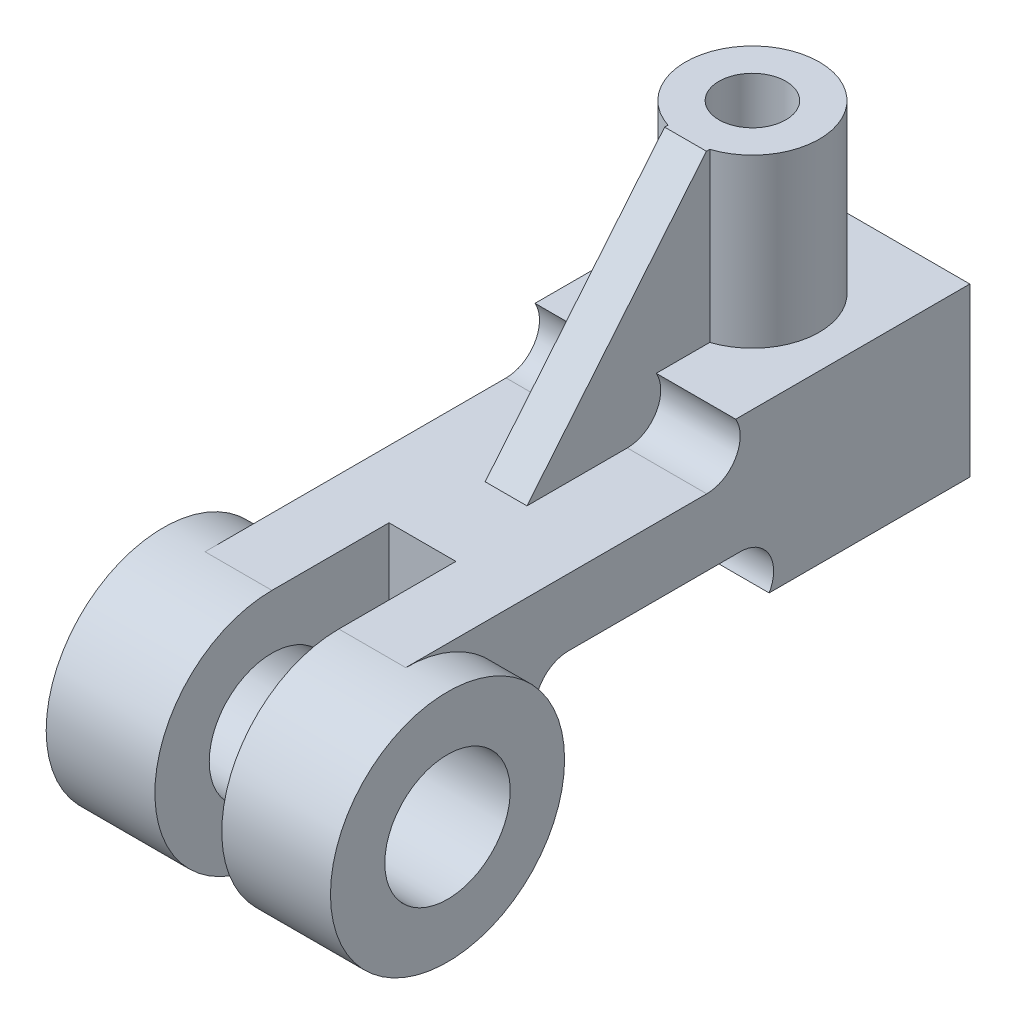
ISO-10303-21;
HEADER;
FILE_DESCRIPTION(('STEP AP214'),'2;1');
FILE_NAME('part.step','',(''),(''),'','','');
FILE_SCHEMA(('AUTOMOTIVE_DESIGN { 1 0 10303 214 1 1 1 1 }'));
ENDSEC;
DATA;
#1=APPLICATION_CONTEXT('core data for automotive mechanical design processes');
#2=APPLICATION_PROTOCOL_DEFINITION('international standard','automotive_design',2000,#1);
#3=PRODUCT_CONTEXT('',#1,'mechanical');
#4=PRODUCT('Part','Part','',(#3));
#5=PRODUCT_RELATED_PRODUCT_CATEGORY('part','',(#4));
#6=PRODUCT_DEFINITION_FORMATION('','',#4);
#7=PRODUCT_DEFINITION_CONTEXT('part definition',#1,'design');
#8=PRODUCT_DEFINITION('design','',#6,#7);
#9=PRODUCT_DEFINITION_SHAPE('','',#8);
#10=(LENGTH_UNIT() NAMED_UNIT(*) SI_UNIT(.MILLI.,.METRE.));
#11=(NAMED_UNIT(*) PLANE_ANGLE_UNIT() SI_UNIT($,.RADIAN.));
#12=(NAMED_UNIT(*) SI_UNIT($,.STERADIAN.) SOLID_ANGLE_UNIT());
#13=UNCERTAINTY_MEASURE_WITH_UNIT(LENGTH_MEASURE(1.E-05),#10,'distance_accuracy_value','');
#14=(GEOMETRIC_REPRESENTATION_CONTEXT(3) GLOBAL_UNCERTAINTY_ASSIGNED_CONTEXT((#13)) GLOBAL_UNIT_ASSIGNED_CONTEXT((#10,
#11,#12)) REPRESENTATION_CONTEXT('',''));
#15=CARTESIAN_POINT('',(0.,0.,0.));
#16=DIRECTION('',(0.,0.,1.));
#17=DIRECTION('',(1.,0.,0.));
#18=AXIS2_PLACEMENT_3D('',#15,#16,#17);
#19=CARTESIAN_POINT('',(-16.,28.,0.));
#20=DIRECTION('',(0.,-1.,0.));
#21=DIRECTION('',(0.,0.,-1.));
#22=AXIS2_PLACEMENT_3D('',#19,#20,#21);
#23=PLANE('',#22);
#24=DIRECTION('',(0.,0.,-1.));
#25=VECTOR('',#24,1.);
#26=CARTESIAN_POINT('',(-3.,28.,-72.0000000000001));
#27=LINE('',#26,#25);
#28=CARTESIAN_POINT('',(-3.,28.,-48.));
#29=VERTEX_POINT('',#28);
#30=CARTESIAN_POINT('',(-3.,28.,-72.0000000000001));
#31=VERTEX_POINT('',#30);
#32=EDGE_CURVE('E205',#29,#31,#27,.T.);
#33=ORIENTED_EDGE('',*,*,#32,.F.);
#34=DIRECTION('',(-1.,0.,0.));
#35=VECTOR('',#34,1.);
#36=CARTESIAN_POINT('',(-3.,28.,-48.));
#37=LINE('',#36,#35);
#38=CARTESIAN_POINT('',(-13.,28.,-48.));
#39=VERTEX_POINT('',#38);
#40=EDGE_CURVE('E199',#29,#39,#37,.T.);
#41=ORIENTED_EDGE('',*,*,#40,.T.);
#42=DIRECTION('',(0.,0.,-1.));
#43=VECTOR('',#42,1.);
#44=CARTESIAN_POINT('',(-13.,28.,-72.0000000000001));
#45=LINE('',#44,#43);
#46=CARTESIAN_POINT('',(-13.,28.,-72.0000000000001));
#47=VERTEX_POINT('',#46);
#48=EDGE_CURVE('E365',#39,#47,#45,.T.);
#49=ORIENTED_EDGE('',*,*,#48,.T.);
#50=DIRECTION('',(1.,0.,0.));
#51=VECTOR('',#50,1.);
#52=CARTESIAN_POINT('',(-16.,28.,-71.9999999999999));
#53=LINE('',#52,#51);
#54=CARTESIAN_POINT('',(-32.,28.,-72.));
#55=VERTEX_POINT('',#54);
#56=EDGE_CURVE('E332',#55,#47,#53,.T.);
#57=ORIENTED_EDGE('',*,*,#56,.F.);
#58=DIRECTION('',(0.,0.,-1.));
#59=VECTOR('',#58,1.);
#60=CARTESIAN_POINT('',(-32.,28.,0.));
#61=LINE('',#60,#59);
#62=CARTESIAN_POINT('',(-32.,28.,0.));
#63=VERTEX_POINT('',#62);
#64=EDGE_CURVE('E264',#63,#55,#61,.T.);
#65=ORIENTED_EDGE('',*,*,#64,.F.);
#66=DIRECTION('',(1.,0.,0.));
#67=VECTOR('',#66,1.);
#68=CARTESIAN_POINT('',(-32.,28.,0.));
#69=LINE('',#68,#67);
#70=CARTESIAN_POINT('',(-16.,28.,0.));
#71=VERTEX_POINT('',#70);
#72=EDGE_CURVE('E272',#63,#71,#69,.T.);
#73=ORIENTED_EDGE('',*,*,#72,.T.);
#74=DIRECTION('',(0.,0.,1.));
#75=VECTOR('',#74,1.);
#76=CARTESIAN_POINT('',(-16.,28.,0.));
#77=LINE('',#76,#75);
#78=CARTESIAN_POINT('',(-16.,28.,-28.));
#79=VERTEX_POINT('',#78);
#80=EDGE_CURVE('E240',#79,#71,#77,.T.);
#81=ORIENTED_EDGE('',*,*,#80,.F.);
#82=DIRECTION('',(-1.,0.,0.));
#83=VECTOR('',#82,1.);
#84=CARTESIAN_POINT('',(-16.,28.,-28.));
#85=LINE('',#84,#83);
#86=CARTESIAN_POINT('',(0.,28.,-28.));
#87=VERTEX_POINT('',#86);
#88=EDGE_CURVE('E233',#87,#79,#85,.T.);
#89=ORIENTED_EDGE('',*,*,#88,.F.);
#90=DIRECTION('',(0.,0.,-1.));
#91=VECTOR('',#90,1.);
#92=CARTESIAN_POINT('',(0.,28.,0.));
#93=LINE('',#92,#91);
#94=CARTESIAN_POINT('',(0.,28.,0.));
#95=VERTEX_POINT('',#94);
#96=EDGE_CURVE('E227',#95,#87,#93,.T.);
#97=ORIENTED_EDGE('',*,*,#96,.F.);
#98=DIRECTION('',(1.,0.,0.));
#99=VECTOR('',#98,1.);
#100=CARTESIAN_POINT('',(-16.,28.,0.));
#101=LINE('',#100,#99);
#102=CARTESIAN_POINT('',(16.,28.,0.));
#103=VERTEX_POINT('',#102);
#104=EDGE_CURVE('E331',#95,#103,#101,.T.);
#105=ORIENTED_EDGE('',*,*,#104,.T.);
#106=DIRECTION('',(0.,0.,-1.));
#107=VECTOR('',#106,1.);
#108=CARTESIAN_POINT('',(16.,28.,0.));
#109=LINE('',#108,#107);
#110=CARTESIAN_POINT('',(16.,28.,-71.9999999999999));
#111=VERTEX_POINT('',#110);
#112=EDGE_CURVE('E288',#103,#111,#109,.T.);
#113=ORIENTED_EDGE('',*,*,#112,.T.);
#114=EDGE_CURVE('E329',#31,#111,#53,.T.);
#115=ORIENTED_EDGE('',*,*,#114,.F.);
#116=EDGE_LOOP('',(#33,#41,#49,#57,#65,#73,#81,#89,#97,#105,#113,#115));
#117=FACE_BOUND('',#116,.T.);
#118=ADVANCED_FACE('F50',(#117),#23,.F.);
#119=CARTESIAN_POINT('',(-16.,36.,-72.));
#120=DIRECTION('',(1.,0.,0.));
#121=DIRECTION('',(0.,0.,-1.));
#122=AXIS2_PLACEMENT_3D('',#119,#120,#121);
#123=CYLINDRICAL_SURFACE('',#122,7.99999999999999);
#124=CARTESIAN_POINT('',(-3.,36.,-72.));
#125=DIRECTION('',(1.,0.,0.));
#126=DIRECTION('',(0.,0.,1.));
#127=AXIS2_PLACEMENT_3D('',#124,#125,#126);
#128=CIRCLE('',#127,8.);
#129=CARTESIAN_POINT('',(-3.,40.,-78.9282032302755));
#130=VERTEX_POINT('',#129);
#131=EDGE_CURVE('E373',#31,#130,#128,.T.);
#132=ORIENTED_EDGE('',*,*,#131,.F.);
#133=ORIENTED_EDGE('',*,*,#114,.T.);
#134=CARTESIAN_POINT('',(16.,36.,-72.));
#135=DIRECTION('',(1.,0.,0.));
#136=DIRECTION('',(0.,0.,-1.));
#137=AXIS2_PLACEMENT_3D('',#134,#135,#136);
#138=CIRCLE('',#137,7.99999999999999);
#139=CARTESIAN_POINT('',(16.,40.,-78.9282032302755));
#140=VERTEX_POINT('',#139);
#141=EDGE_CURVE('E291',#111,#140,#138,.T.);
#142=ORIENTED_EDGE('',*,*,#141,.T.);
#143=DIRECTION('',(1.,0.,0.));
#144=VECTOR('',#143,1.);
#145=CARTESIAN_POINT('',(-16.,40.,-78.9282032302755));
#146=LINE('',#145,#144);
#147=EDGE_CURVE('E326',#130,#140,#146,.T.);
#148=ORIENTED_EDGE('',*,*,#147,.F.);
#149=EDGE_LOOP('',(#132,#133,#142,#148));
#150=FACE_BOUND('',#149,.T.);
#151=ADVANCED_FACE('F379',(#150),#123,.F.);
#152=CARTESIAN_POINT('',(-16.,40.,-78.9282032302755));
#153=DIRECTION('',(0.,-1.,0.));
#154=DIRECTION('',(0.,0.,-1.));
#155=AXIS2_PLACEMENT_3D('',#152,#153,#154);
#156=PLANE('',#155);
#157=DIRECTION('',(0.,0.,-1.));
#158=VECTOR('',#157,1.);
#159=CARTESIAN_POINT('',(-3.,40.,-93.4436906240122));
#160=LINE('',#159,#158);
#161=CARTESIAN_POINT('',(-3.,40.,-91.7295190767049));
#162=VERTEX_POINT('',#161);
#163=EDGE_CURVE('E211',#130,#162,#160,.T.);
#164=ORIENTED_EDGE('',*,*,#163,.F.);
#165=ORIENTED_EDGE('',*,*,#147,.T.);
#166=DIRECTION('',(0.,0.,-1.));
#167=VECTOR('',#166,1.);
#168=CARTESIAN_POINT('',(16.,40.,-78.9282032302755));
#169=LINE('',#168,#167);
#170=CARTESIAN_POINT('',(16.,40.,-134.928203230276));
#171=VERTEX_POINT('',#170);
#172=EDGE_CURVE('E298',#140,#171,#169,.T.);
#173=ORIENTED_EDGE('',*,*,#172,.T.);
#174=DIRECTION('',(1.,0.,0.));
#175=VECTOR('',#174,1.);
#176=CARTESIAN_POINT('',(-32.,40.,-134.928203230276));
#177=LINE('',#176,#175);
#178=CARTESIAN_POINT('',(-32.,40.,-134.928203230276));
#179=VERTEX_POINT('',#178);
#180=EDGE_CURVE('E224',#179,#171,#177,.T.);
#181=ORIENTED_EDGE('',*,*,#180,.F.);
#182=DIRECTION('',(0.,0.,1.));
#183=VECTOR('',#182,1.);
#184=CARTESIAN_POINT('',(-32.,40.,0.));
#185=LINE('',#184,#183);
#186=CARTESIAN_POINT('',(-32.,40.,-78.9282032302755));
#187=VERTEX_POINT('',#186);
#188=EDGE_CURVE('E257',#179,#187,#185,.T.);
#189=ORIENTED_EDGE('',*,*,#188,.T.);
#190=CARTESIAN_POINT('',(-13.,40.,-78.9282032302755));
#191=VERTEX_POINT('',#190);
#192=EDGE_CURVE('E330',#187,#191,#146,.T.);
#193=ORIENTED_EDGE('',*,*,#192,.T.);
#194=DIRECTION('',(0.,0.,-1.));
#195=VECTOR('',#194,1.);
#196=CARTESIAN_POINT('',(-13.,40.,-93.4436906240122));
#197=LINE('',#196,#195);
#198=CARTESIAN_POINT('',(-13.,40.,-91.7295190767049));
#199=VERTEX_POINT('',#198);
#200=EDGE_CURVE('E193',#191,#199,#197,.T.);
#201=ORIENTED_EDGE('',*,*,#200,.T.);
#202=CARTESIAN_POINT('',(-8.,40.,-106.928203230276));
#203=DIRECTION('',(0.,-1.,0.));
#204=DIRECTION('',(0.,0.,-1.));
#205=AXIS2_PLACEMENT_3D('',#202,#203,#204);
#206=CIRCLE('',#205,16.);
#207=EDGE_CURVE('E348',#162,#199,#206,.F.);
#208=ORIENTED_EDGE('',*,*,#207,.F.);
#209=EDGE_LOOP('',(#164,#165,#173,#181,#189,#193,#201,#208));
#210=FACE_BOUND('',#209,.T.);
#211=ADVANCED_FACE('F363',(#210),#156,.F.);
#212=CARTESIAN_POINT('',(-8.,80.,-106.928203230276));
#213=DIRECTION('',(0.,-1.,0.));
#214=DIRECTION('',(0.,0.,-1.));
#215=AXIS2_PLACEMENT_3D('',#212,#213,#214);
#216=CYLINDRICAL_SURFACE('',#215,16.);
#217=DIRECTION('',(0.,-1.,0.));
#218=VECTOR('',#217,1.);
#219=CARTESIAN_POINT('',(-3.,80.,-91.7295190767049));
#220=LINE('',#219,#218);
#221=CARTESIAN_POINT('',(-3.,80.,-91.7295190767049));
#222=VERTEX_POINT('',#221);
#223=EDGE_CURVE('E11',#162,#222,#220,.F.);
#224=ORIENTED_EDGE('',*,*,#223,.F.);
#225=ORIENTED_EDGE('',*,*,#207,.T.);
#226=DIRECTION('',(0.,-1.,0.));
#227=VECTOR('',#226,1.);
#228=CARTESIAN_POINT('',(-13.,80.,-91.7295190767049));
#229=LINE('',#228,#227);
#230=CARTESIAN_POINT('',(-13.,80.,-91.7295190767049));
#231=VERTEX_POINT('',#230);
#232=EDGE_CURVE('E54',#199,#231,#229,.F.);
#233=ORIENTED_EDGE('',*,*,#232,.T.);
#234=CARTESIAN_POINT('',(-8.,80.,-106.928203230276));
#235=DIRECTION('',(0.,1.,0.));
#236=DIRECTION('',(0.,0.,1.));
#237=AXIS2_PLACEMENT_3D('',#234,#235,#236);
#238=CIRCLE('',#237,16.);
#239=EDGE_CURVE('E220',#222,#231,#238,.T.);
#240=ORIENTED_EDGE('',*,*,#239,.F.);
#241=EDGE_LOOP('',(#224,#225,#233,#240));
#242=FACE_BOUND('',#241,.T.);
#243=ADVANCED_FACE('F352',(#242),#216,.T.);
#244=CARTESIAN_POINT('',(26.,0.,0.));
#245=DIRECTION('',(-1.,0.,0.));
#246=DIRECTION('',(0.,0.,1.));
#247=AXIS2_PLACEMENT_3D('',#244,#245,#246);
#248=CYLINDRICAL_SURFACE('',#247,15.);
#249=CARTESIAN_POINT('',(0.,0.,0.));
#250=DIRECTION('',(1.,0.,0.));
#251=DIRECTION('',(0.,0.,-1.));
#252=AXIS2_PLACEMENT_3D('',#249,#250,#251);
#253=CIRCLE('',#252,15.);
#254=CARTESIAN_POINT('',(0.,0.,15.));
#255=VERTEX_POINT('',#254);
#256=EDGE_CURVE('E339',#255,#255,#253,.T.);
#257=CARTESIAN_POINT('',(26.,0.,0.));
#258=DIRECTION('',(1.,0.,0.));
#259=DIRECTION('',(0.,0.,-1.));
#260=AXIS2_PLACEMENT_3D('',#257,#258,#259);
#261=CIRCLE('',#260,15.);
#262=CARTESIAN_POINT('',(26.,0.,15.));
#263=VERTEX_POINT('',#262);
#264=EDGE_CURVE('E341',#263,#263,#261,.T.);
#265=CARTESIAN_POINT('',(0.,0.,15.));
#266=CARTESIAN_POINT('',(0.270833333333333,0.,15.));
#267=CARTESIAN_POINT('',(0.541666666666667,0.,15.));
#268=CARTESIAN_POINT('',(1.08333333333333,0.,15.));
#269=CARTESIAN_POINT('',(1.35416666666667,0.,15.));
#270=CARTESIAN_POINT('',(1.89583333333333,0.,15.));
#271=CARTESIAN_POINT('',(2.16666666666667,0.,15.));
#272=CARTESIAN_POINT('',(2.70833333333333,0.,15.));
#273=CARTESIAN_POINT('',(2.97916666666667,0.,15.));
#274=CARTESIAN_POINT('',(3.52083333333333,0.,15.));
#275=CARTESIAN_POINT('',(3.79166666666667,0.,15.));
#276=CARTESIAN_POINT('',(4.33333333333333,0.,15.));
#277=CARTESIAN_POINT('',(4.60416666666667,0.,15.));
#278=CARTESIAN_POINT('',(5.14583333333333,0.,15.));
#279=CARTESIAN_POINT('',(5.41666666666667,0.,15.));
#280=CARTESIAN_POINT('',(5.95833333333333,0.,15.));
#281=CARTESIAN_POINT('',(6.22916666666667,0.,15.));
#282=CARTESIAN_POINT('',(6.77083333333333,0.,15.));
#283=CARTESIAN_POINT('',(7.04166666666667,0.,15.));
#284=CARTESIAN_POINT('',(7.58333333333333,0.,15.));
#285=CARTESIAN_POINT('',(7.85416666666667,0.,15.));
#286=CARTESIAN_POINT('',(8.39583333333333,0.,15.));
#287=CARTESIAN_POINT('',(8.66666666666667,0.,15.));
#288=CARTESIAN_POINT('',(9.20833333333333,0.,15.));
#289=CARTESIAN_POINT('',(9.47916666666667,0.,15.));
#290=CARTESIAN_POINT('',(10.0208333333333,0.,15.));
#291=CARTESIAN_POINT('',(10.2916666666667,0.,15.));
#292=CARTESIAN_POINT('',(10.8333333333333,0.,15.));
#293=CARTESIAN_POINT('',(11.1041666666667,0.,15.));
#294=CARTESIAN_POINT('',(11.6458333333333,0.,15.));
#295=CARTESIAN_POINT('',(11.9166666666667,0.,15.));
#296=CARTESIAN_POINT('',(12.4583333333333,0.,15.));
#297=CARTESIAN_POINT('',(12.7291666666667,0.,15.));
#298=CARTESIAN_POINT('',(13.2708333333333,0.,15.));
#299=CARTESIAN_POINT('',(13.5416666666667,0.,15.));
#300=CARTESIAN_POINT('',(14.0833333333333,0.,15.));
#301=CARTESIAN_POINT('',(14.3541666666667,0.,15.));
#302=CARTESIAN_POINT('',(14.8958333333333,0.,15.));
#303=CARTESIAN_POINT('',(15.1666666666667,0.,15.));
#304=CARTESIAN_POINT('',(15.7083333333333,0.,15.));
#305=CARTESIAN_POINT('',(15.9791666666667,0.,15.));
#306=CARTESIAN_POINT('',(16.5208333333333,0.,15.));
#307=CARTESIAN_POINT('',(16.7916666666667,0.,15.));
#308=CARTESIAN_POINT('',(17.3333333333333,0.,15.));
#309=CARTESIAN_POINT('',(17.6041666666667,0.,15.));
#310=CARTESIAN_POINT('',(18.1458333333333,0.,15.));
#311=CARTESIAN_POINT('',(18.4166666666667,0.,15.));
#312=CARTESIAN_POINT('',(18.9583333333333,0.,15.));
#313=CARTESIAN_POINT('',(19.2291666666667,0.,15.));
#314=CARTESIAN_POINT('',(19.7708333333333,0.,15.));
#315=CARTESIAN_POINT('',(20.0416666666667,0.,15.));
#316=CARTESIAN_POINT('',(20.5833333333333,0.,15.));
#317=CARTESIAN_POINT('',(20.8541666666667,0.,15.));
#318=CARTESIAN_POINT('',(21.3958333333333,0.,15.));
#319=CARTESIAN_POINT('',(21.6666666666667,0.,15.));
#320=CARTESIAN_POINT('',(22.2083333333333,0.,15.));
#321=CARTESIAN_POINT('',(22.4791666666667,0.,15.));
#322=CARTESIAN_POINT('',(23.0208333333333,0.,15.));
#323=CARTESIAN_POINT('',(23.2916666666667,0.,15.));
#324=CARTESIAN_POINT('',(23.8333333333333,0.,15.));
#325=CARTESIAN_POINT('',(24.1041666666667,0.,15.));
#326=CARTESIAN_POINT('',(24.6458333333333,0.,15.));
#327=CARTESIAN_POINT('',(24.9166666666667,0.,15.));
#328=CARTESIAN_POINT('',(25.4583333333333,0.,15.));
#329=CARTESIAN_POINT('',(25.7291666666667,0.,15.));
#330=CARTESIAN_POINT('',(26.,0.,15.));
#331=B_SPLINE_CURVE_WITH_KNOTS('',3,(#265,#266,#267,#268,#269,#270,#271,#272,#273,#274,#275,
#276,#277,#278,#279,#280,#281,#282,#283,#284,#285,#286,#287,#288,#289,#290,#291,#292,#293,#294,
#295,#296,#297,#298,#299,#300,#301,#302,#303,#304,#305,#306,#307,#308,#309,#310,#311,#312,#313,
#314,#315,#316,#317,#318,#319,#320,#321,#322,#323,#324,#325,#326,#327,#328,#329,#330),
.UNSPECIFIED.,.F.,.F.,(4,2,2,2,2,2,2,2,2,2,2,2,2,2,2,2,2,2,2,2,2,2,2,2,2,2,2,2,2,2,2,2,4),(0.,
0.812500000000001,1.625,2.4375,3.25,4.0625,4.875,5.6875,6.5,7.3125,8.125,8.9375,9.75,10.5625,
11.375,12.1875,13.,13.8125,14.625,15.4375,16.25,17.0625,17.875,18.6875,19.5,20.3125,21.125,
21.9375,22.75,23.5625,24.375,25.1875,26.),.UNSPECIFIED.);
#332=EDGE_CURVE('BSEAM462',#255,#263,#331,.T.);
#333=ORIENTED_EDGE('',*,*,#256,.F.);
#334=ORIENTED_EDGE('',*,*,#264,.T.);
#335=ORIENTED_EDGE('',*,*,#332,.T.);
#336=ORIENTED_EDGE('',*,*,#332,.F.);
#337=EDGE_LOOP('',(#333,#335,#334,#336));
#338=FACE_BOUND('',#337,.T.);
#339=ADVANCED_FACE('F462',(#338),#248,.F.);
#340=CARTESIAN_POINT('',(0.,0.,0.));
#341=DIRECTION('',(1.,0.,0.));
#342=DIRECTION('',(0.,0.,-1.));
#343=AXIS2_PLACEMENT_3D('',#340,#341,#342);
#344=PLANE('',#343);
#345=DIRECTION('',(0.,1.,0.));
#346=VECTOR('',#345,1.);
#347=CARTESIAN_POINT('',(0.,-4.,-28.));
#348=LINE('',#347,#346);
#349=CARTESIAN_POINT('',(0.,0.,-28.));
#350=VERTEX_POINT('',#349);
#351=EDGE_CURVE('E239',#350,#87,#348,.T.);
#352=ORIENTED_EDGE('',*,*,#351,.F.);
#353=CARTESIAN_POINT('',(0.,0.,0.));
#354=DIRECTION('',(1.,0.,0.));
#355=DIRECTION('',(0.,0.,-1.));
#356=AXIS2_PLACEMENT_3D('',#353,#354,#355);
#357=CIRCLE('',#356,28.);
#358=EDGE_CURVE('E343',#95,#350,#357,.T.);
#359=ORIENTED_EDGE('',*,*,#358,.F.);
#360=ORIENTED_EDGE('',*,*,#96,.T.);
#361=EDGE_LOOP('',(#352,#359,#360));
#362=FACE_BOUND('',#361,.T.);
#363=ORIENTED_EDGE('',*,*,#256,.T.);
#364=EDGE_LOOP('',(#363));
#365=FACE_BOUND('',#364,.T.);
#366=ADVANCED_FACE('F423',(#362,#365),#344,.F.);
#367=CARTESIAN_POINT('',(26.,0.,0.));
#368=DIRECTION('',(1.,0.,0.));
#369=DIRECTION('',(0.,0.,-1.));
#370=AXIS2_PLACEMENT_3D('',#367,#368,#369);
#371=PLANE('',#370);
#372=CARTESIAN_POINT('',(26.,0.,0.));
#373=DIRECTION('',(1.,0.,0.));
#374=DIRECTION('',(0.,0.,-1.));
#375=AXIS2_PLACEMENT_3D('',#372,#373,#374);
#376=CIRCLE('',#375,28.);
#377=CARTESIAN_POINT('',(26.,0.,-28.));
#378=VERTEX_POINT('',#377);
#379=EDGE_CURVE('E350',#378,#378,#376,.T.);
#380=ORIENTED_EDGE('',*,*,#379,.T.);
#381=EDGE_LOOP('',(#380));
#382=FACE_BOUND('',#381,.T.);
#383=ORIENTED_EDGE('',*,*,#264,.F.);
#384=EDGE_LOOP('',(#383));
#385=FACE_BOUND('',#384,.T.);
#386=ADVANCED_FACE('F464',(#382,#385),#371,.T.);
#387=CARTESIAN_POINT('',(26.,0.,0.));
#388=DIRECTION('',(-1.,0.,0.));
#389=DIRECTION('',(0.,0.,1.));
#390=AXIS2_PLACEMENT_3D('',#387,#388,#389);
#391=CYLINDRICAL_SURFACE('',#390,28.);
#392=CARTESIAN_POINT('',(16.,0.,0.));
#393=DIRECTION('',(-1.,0.,0.));
#394=DIRECTION('',(0.,0.,1.));
#395=AXIS2_PLACEMENT_3D('',#392,#393,#394);
#396=CIRCLE('',#395,28.);
#397=CARTESIAN_POINT('',(16.,0.,-28.));
#398=VERTEX_POINT('',#397);
#399=EDGE_CURVE('E69',#103,#398,#396,.T.);
#400=ORIENTED_EDGE('',*,*,#399,.F.);
#401=ORIENTED_EDGE('',*,*,#104,.F.);
#402=ORIENTED_EDGE('',*,*,#358,.T.);
#403=DIRECTION('',(-1.,0.,0.));
#404=VECTOR('',#403,1.);
#405=CARTESIAN_POINT('',(26.,0.,-28.));
#406=LINE('',#405,#404);
#407=EDGE_CURVE('E340',#398,#350,#406,.T.);
#408=ORIENTED_EDGE('',*,*,#407,.F.);
#409=EDGE_LOOP('',(#400,#401,#402,#408));
#410=FACE_BOUND('',#409,.T.);
#411=ORIENTED_EDGE('',*,*,#379,.F.);
#412=EDGE_LOOP('',(#411));
#413=FACE_BOUND('',#412,.T.);
#414=ADVANCED_FACE('F47',(#410,#413),#391,.T.);
#415=CARTESIAN_POINT('',(-16.,0.,0.));
#416=DIRECTION('',(1.,0.,0.));
#417=DIRECTION('',(0.,0.,-1.));
#418=AXIS2_PLACEMENT_3D('',#415,#416,#417);
#419=CIRCLE('',#418,15.);
#420=CARTESIAN_POINT('',(-16.,0.,15.));
#421=VERTEX_POINT('',#420);
#422=EDGE_CURVE('E280',#421,#421,#419,.T.);
#423=CARTESIAN_POINT('',(-42.,0.,0.));
#424=DIRECTION('',(1.,0.,0.));
#425=DIRECTION('',(0.,0.,-1.));
#426=AXIS2_PLACEMENT_3D('',#423,#424,#425);
#427=CIRCLE('',#426,15.);
#428=CARTESIAN_POINT('',(-42.,0.,15.));
#429=VERTEX_POINT('',#428);
#430=EDGE_CURVE('E278',#429,#429,#427,.T.);
#431=CARTESIAN_POINT('',(-16.,0.,15.));
#432=CARTESIAN_POINT('',(-16.2708333333333,0.,15.));
#433=CARTESIAN_POINT('',(-16.5416666666667,0.,15.));
#434=CARTESIAN_POINT('',(-17.0833333333333,0.,15.));
#435=CARTESIAN_POINT('',(-17.3541666666667,0.,15.));
#436=CARTESIAN_POINT('',(-17.8958333333333,0.,15.));
#437=CARTESIAN_POINT('',(-18.1666666666667,0.,15.));
#438=CARTESIAN_POINT('',(-18.7083333333333,0.,15.));
#439=CARTESIAN_POINT('',(-18.9791666666667,0.,15.));
#440=CARTESIAN_POINT('',(-19.5208333333333,0.,15.));
#441=CARTESIAN_POINT('',(-19.7916666666667,0.,15.));
#442=CARTESIAN_POINT('',(-20.3333333333333,0.,15.));
#443=CARTESIAN_POINT('',(-20.6041666666667,0.,15.));
#444=CARTESIAN_POINT('',(-21.1458333333333,0.,15.));
#445=CARTESIAN_POINT('',(-21.4166666666667,0.,15.));
#446=CARTESIAN_POINT('',(-21.9583333333333,0.,15.));
#447=CARTESIAN_POINT('',(-22.2291666666667,0.,15.));
#448=CARTESIAN_POINT('',(-22.7708333333333,0.,15.));
#449=CARTESIAN_POINT('',(-23.0416666666667,0.,15.));
#450=CARTESIAN_POINT('',(-23.5833333333333,0.,15.));
#451=CARTESIAN_POINT('',(-23.8541666666667,0.,15.));
#452=CARTESIAN_POINT('',(-24.3958333333333,0.,15.));
#453=CARTESIAN_POINT('',(-24.6666666666667,0.,15.));
#454=CARTESIAN_POINT('',(-25.2083333333333,0.,15.));
#455=CARTESIAN_POINT('',(-25.4791666666667,0.,15.));
#456=CARTESIAN_POINT('',(-26.0208333333333,0.,15.));
#457=CARTESIAN_POINT('',(-26.2916666666667,0.,15.));
#458=CARTESIAN_POINT('',(-26.8333333333333,0.,15.));
#459=CARTESIAN_POINT('',(-27.1041666666667,0.,15.));
#460=CARTESIAN_POINT('',(-27.6458333333333,0.,15.));
#461=CARTESIAN_POINT('',(-27.9166666666667,0.,15.));
#462=CARTESIAN_POINT('',(-28.4583333333333,0.,15.));
#463=CARTESIAN_POINT('',(-28.7291666666667,0.,15.));
#464=CARTESIAN_POINT('',(-29.2708333333333,0.,15.));
#465=CARTESIAN_POINT('',(-29.5416666666667,0.,15.));
#466=CARTESIAN_POINT('',(-30.0833333333333,0.,15.));
#467=CARTESIAN_POINT('',(-30.3541666666667,0.,15.));
#468=CARTESIAN_POINT('',(-30.8958333333333,0.,15.));
#469=CARTESIAN_POINT('',(-31.1666666666667,0.,15.));
#470=CARTESIAN_POINT('',(-31.7083333333333,0.,15.));
#471=CARTESIAN_POINT('',(-31.9791666666667,0.,15.));
#472=CARTESIAN_POINT('',(-32.5208333333333,0.,15.));
#473=CARTESIAN_POINT('',(-32.7916666666667,0.,15.));
#474=CARTESIAN_POINT('',(-33.3333333333333,0.,15.));
#475=CARTESIAN_POINT('',(-33.6041666666667,0.,15.));
#476=CARTESIAN_POINT('',(-34.1458333333333,0.,15.));
#477=CARTESIAN_POINT('',(-34.4166666666667,0.,15.));
#478=CARTESIAN_POINT('',(-34.9583333333333,0.,15.));
#479=CARTESIAN_POINT('',(-35.2291666666667,0.,15.));
#480=CARTESIAN_POINT('',(-35.7708333333333,0.,15.));
#481=CARTESIAN_POINT('',(-36.0416666666667,0.,15.));
#482=CARTESIAN_POINT('',(-36.5833333333333,0.,15.));
#483=CARTESIAN_POINT('',(-36.8541666666667,0.,15.));
#484=CARTESIAN_POINT('',(-37.3958333333333,0.,15.));
#485=CARTESIAN_POINT('',(-37.6666666666667,0.,15.));
#486=CARTESIAN_POINT('',(-38.2083333333333,0.,15.));
#487=CARTESIAN_POINT('',(-38.4791666666667,0.,15.));
#488=CARTESIAN_POINT('',(-39.0208333333333,0.,15.));
#489=CARTESIAN_POINT('',(-39.2916666666667,0.,15.));
#490=CARTESIAN_POINT('',(-39.8333333333333,0.,15.));
#491=CARTESIAN_POINT('',(-40.1041666666667,0.,15.));
#492=CARTESIAN_POINT('',(-40.6458333333333,0.,15.));
#493=CARTESIAN_POINT('',(-40.9166666666667,0.,15.));
#494=CARTESIAN_POINT('',(-41.4583333333333,0.,15.));
#495=CARTESIAN_POINT('',(-41.7291666666667,0.,15.));
#496=CARTESIAN_POINT('',(-42.,0.,15.));
#497=B_SPLINE_CURVE_WITH_KNOTS('',3,(#431,#432,#433,#434,#435,#436,#437,#438,#439,#440,#441,
#442,#443,#444,#445,#446,#447,#448,#449,#450,#451,#452,#453,#454,#455,#456,#457,#458,#459,#460,
#461,#462,#463,#464,#465,#466,#467,#468,#469,#470,#471,#472,#473,#474,#475,#476,#477,#478,#479,
#480,#481,#482,#483,#484,#485,#486,#487,#488,#489,#490,#491,#492,#493,#494,#495,#496),
.UNSPECIFIED.,.F.,.F.,(4,2,2,2,2,2,2,2,2,2,2,2,2,2,2,2,2,2,2,2,2,2,2,2,2,2,2,2,2,2,2,2,4),(0.,
0.812500000000001,1.625,2.4375,3.25,4.0625,4.875,5.6875,6.5,7.3125,8.125,8.9375,
9.74999999999999,10.5625,11.375,12.1875,13.,13.8125,14.625,15.4375,16.25,17.0625,17.875,18.6875,
19.5,20.3125,21.125,21.9375,22.75,23.5625,24.375,25.1875,26.),.UNSPECIFIED.);
#498=EDGE_CURVE('BSEAM458',#421,#429,#497,.T.);
#499=ORIENTED_EDGE('',*,*,#422,.T.);
#500=ORIENTED_EDGE('',*,*,#430,.F.);
#501=ORIENTED_EDGE('',*,*,#498,.T.);
#502=ORIENTED_EDGE('',*,*,#498,.F.);
#503=EDGE_LOOP('',(#499,#501,#500,#502));
#504=FACE_BOUND('',#503,.T.);
#505=ADVANCED_FACE('F458',(#504),#248,.F.);
#506=CARTESIAN_POINT('',(-16.,0.,-15.));
#507=DIRECTION('',(0.,1.,0.));
#508=DIRECTION('',(0.,0.,1.));
#509=AXIS2_PLACEMENT_3D('',#506,#507,#508);
#510=PLANE('',#509);
#511=ORIENTED_EDGE('',*,*,#407,.T.);
#512=DIRECTION('',(-1.,0.,0.));
#513=VECTOR('',#512,1.);
#514=CARTESIAN_POINT('',(-16.,0.,-28.));
#515=LINE('',#514,#513);
#516=CARTESIAN_POINT('',(-16.,0.,-28.));
#517=VERTEX_POINT('',#516);
#518=EDGE_CURVE('E245',#350,#517,#515,.T.);
#519=ORIENTED_EDGE('',*,*,#518,.T.);
#520=DIRECTION('',(1.,0.,0.));
#521=VECTOR('',#520,1.);
#522=CARTESIAN_POINT('',(-32.,0.,-28.));
#523=LINE('',#522,#521);
#524=CARTESIAN_POINT('',(-32.,0.,-28.));
#525=VERTEX_POINT('',#524);
#526=EDGE_CURVE('E273',#525,#517,#523,.T.);
#527=ORIENTED_EDGE('',*,*,#526,.F.);
#528=DIRECTION('',(0.,0.,-1.));
#529=VECTOR('',#528,1.);
#530=CARTESIAN_POINT('',(-32.,0.,0.));
#531=LINE('',#530,#529);
#532=CARTESIAN_POINT('',(-32.,0.,-30.9282032302755));
#533=VERTEX_POINT('',#532);
#534=EDGE_CURVE('E269',#525,#533,#531,.T.);
#535=ORIENTED_EDGE('',*,*,#534,.T.);
#536=DIRECTION('',(1.,0.,0.));
#537=VECTOR('',#536,1.);
#538=CARTESIAN_POINT('',(-16.,0.,-30.9282032302755));
#539=LINE('',#538,#537);
#540=CARTESIAN_POINT('',(16.,0.,-30.9282032302755));
#541=VERTEX_POINT('',#540);
#542=EDGE_CURVE('E313',#533,#541,#539,.T.);
#543=ORIENTED_EDGE('',*,*,#542,.T.);
#544=DIRECTION('',(0.,0.,1.));
#545=VECTOR('',#544,1.);
#546=CARTESIAN_POINT('',(16.,0.,-15.));
#547=LINE('',#546,#545);
#548=EDGE_CURVE('E306',#541,#398,#547,.T.);
#549=ORIENTED_EDGE('',*,*,#548,.T.);
#550=EDGE_LOOP('',(#511,#519,#527,#535,#543,#549));
#551=FACE_BOUND('',#550,.T.);
#552=ADVANCED_FACE('F430',(#551),#510,.F.);
#553=CARTESIAN_POINT('',(16.,0.,0.));
#554=DIRECTION('',(-1.,0.,0.));
#555=DIRECTION('',(0.,0.,1.));
#556=AXIS2_PLACEMENT_3D('',#553,#554,#555);
#557=PLANE('',#556);
#558=CARTESIAN_POINT('',(16.,3.99999999999998,-80.));
#559=DIRECTION('',(1.,0.,0.));
#560=DIRECTION('',(0.,0.,-1.));
#561=AXIS2_PLACEMENT_3D('',#558,#559,#560);
#562=CIRCLE('',#561,8.00000000000003);
#563=CARTESIAN_POINT('',(16.,0.,-86.9282032302755));
#564=VERTEX_POINT('',#563);
#565=CARTESIAN_POINT('',(16.,12.,-80.));
#566=VERTEX_POINT('',#565);
#567=EDGE_CURVE('E299',#564,#566,#562,.T.);
#568=ORIENTED_EDGE('',*,*,#567,.F.);
#569=DIRECTION('',(0.,0.,1.));
#570=VECTOR('',#569,1.);
#571=CARTESIAN_POINT('',(16.,0.,-114.928203230276));
#572=LINE('',#571,#570);
#573=CARTESIAN_POINT('',(16.,0.,-134.928203230276));
#574=VERTEX_POINT('',#573);
#575=EDGE_CURVE('E296',#574,#564,#572,.T.);
#576=ORIENTED_EDGE('',*,*,#575,.F.);
#577=DIRECTION('',(0.,1.,0.));
#578=VECTOR('',#577,1.);
#579=CARTESIAN_POINT('',(16.,40.,-134.928203230276));
#580=LINE('',#579,#578);
#581=EDGE_CURVE('E218',#574,#171,#580,.T.);
#582=ORIENTED_EDGE('',*,*,#581,.T.);
#583=ORIENTED_EDGE('',*,*,#172,.F.);
#584=ORIENTED_EDGE('',*,*,#141,.F.);
#585=ORIENTED_EDGE('',*,*,#112,.F.);
#586=ORIENTED_EDGE('',*,*,#399,.T.);
#587=ORIENTED_EDGE('',*,*,#548,.F.);
#588=DIRECTION('',(0.,-1.,0.));
#589=VECTOR('',#588,1.);
#590=CARTESIAN_POINT('',(16.,0.,-30.9282032302755));
#591=LINE('',#590,#589);
#592=CARTESIAN_POINT('',(16.,3.99999999999995,-30.9282032302755));
#593=VERTEX_POINT('',#592);
#594=EDGE_CURVE('E308',#593,#541,#591,.T.);
#595=ORIENTED_EDGE('',*,*,#594,.F.);
#596=CARTESIAN_POINT('',(16.,3.99999999999999,-38.9282032302755));
#597=DIRECTION('',(1.,0.,0.));
#598=DIRECTION('',(0.,0.,-1.));
#599=AXIS2_PLACEMENT_3D('',#596,#597,#598);
#600=CIRCLE('',#599,8.00000000000001);
#601=CARTESIAN_POINT('',(16.,12.,-38.9282032302756));
#602=VERTEX_POINT('',#601);
#603=EDGE_CURVE('E303',#602,#593,#600,.T.);
#604=ORIENTED_EDGE('',*,*,#603,.F.);
#605=DIRECTION('',(0.,0.,1.));
#606=VECTOR('',#605,1.);
#607=CARTESIAN_POINT('',(16.,12.,-80.));
#608=LINE('',#607,#606);
#609=EDGE_CURVE('E305',#566,#602,#608,.T.);
#610=ORIENTED_EDGE('',*,*,#609,.F.);
#611=EDGE_LOOP('',(#568,#576,#582,#583,#584,#585,#586,#587,#595,#604,#610));
#612=FACE_BOUND('',#611,.T.);
#613=ADVANCED_FACE('F387',(#612),#557,.F.);
#614=ORIENTED_EDGE('',*,*,#56,.T.);
#615=CARTESIAN_POINT('',(-13.,36.,-72.));
#616=DIRECTION('',(1.,0.,0.));
#617=DIRECTION('',(0.,0.,1.));
#618=AXIS2_PLACEMENT_3D('',#615,#616,#617);
#619=CIRCLE('',#618,8.);
#620=EDGE_CURVE('E361',#47,#191,#619,.T.);
#621=ORIENTED_EDGE('',*,*,#620,.T.);
#622=ORIENTED_EDGE('',*,*,#192,.F.);
#623=CARTESIAN_POINT('',(-32.,36.,-72.));
#624=DIRECTION('',(1.,0.,0.));
#625=DIRECTION('',(0.,0.,-1.));
#626=AXIS2_PLACEMENT_3D('',#623,#624,#625);
#627=CIRCLE('',#626,8.);
#628=EDGE_CURVE('E265',#187,#55,#627,.F.);
#629=ORIENTED_EDGE('',*,*,#628,.T.);
#630=EDGE_LOOP('',(#614,#621,#622,#629));
#631=FACE_BOUND('',#630,.T.);
#632=ADVANCED_FACE('F398',(#631),#123,.F.);
#633=CARTESIAN_POINT('',(-16.,0.,-114.928203230276));
#634=DIRECTION('',(0.,1.,0.));
#635=DIRECTION('',(0.,0.,1.));
#636=AXIS2_PLACEMENT_3D('',#633,#634,#635);
#637=PLANE('',#636);
#638=CARTESIAN_POINT('',(-8.,0.,-106.928203230276));
#639=DIRECTION('',(0.,1.,0.));
#640=DIRECTION('',(0.,0.,1.));
#641=AXIS2_PLACEMENT_3D('',#638,#639,#640);
#642=CIRCLE('',#641,8.00000000000001);
#643=CARTESIAN_POINT('',(-8.,0.,-98.9282032302755));
#644=VERTEX_POINT('',#643);
#645=EDGE_CURVE('E206',#644,#644,#642,.T.);
#646=ORIENTED_EDGE('',*,*,#645,.T.);
#647=EDGE_LOOP('',(#646));
#648=FACE_BOUND('',#647,.T.);
#649=DIRECTION('',(1.,0.,0.));
#650=VECTOR('',#649,1.);
#651=CARTESIAN_POINT('',(-16.,0.,-86.9282032302755));
#652=LINE('',#651,#650);
#653=CARTESIAN_POINT('',(-32.,0.,-86.9282032302755));
#654=VERTEX_POINT('',#653);
#655=EDGE_CURVE('E323',#654,#564,#652,.T.);
#656=ORIENTED_EDGE('',*,*,#655,.F.);
#657=DIRECTION('',(0.,0.,1.));
#658=VECTOR('',#657,1.);
#659=CARTESIAN_POINT('',(-32.,0.,0.));
#660=LINE('',#659,#658);
#661=CARTESIAN_POINT('',(-32.,0.,-134.928203230276));
#662=VERTEX_POINT('',#661);
#663=EDGE_CURVE('E256',#662,#654,#660,.T.);
#664=ORIENTED_EDGE('',*,*,#663,.F.);
#665=DIRECTION('',(1.,0.,0.));
#666=VECTOR('',#665,1.);
#667=CARTESIAN_POINT('',(-32.,0.,-134.928203230276));
#668=LINE('',#667,#666);
#669=EDGE_CURVE('E228',#662,#574,#668,.T.);
#670=ORIENTED_EDGE('',*,*,#669,.T.);
#671=ORIENTED_EDGE('',*,*,#575,.T.);
#672=EDGE_LOOP('',(#656,#664,#670,#671));
#673=FACE_BOUND('',#672,.T.);
#674=ADVANCED_FACE('F442',(#648,#673),#637,.F.);
#675=CARTESIAN_POINT('',(-16.,3.99999999999998,-80.));
#676=DIRECTION('',(1.,0.,0.));
#677=DIRECTION('',(0.,0.,-1.));
#678=AXIS2_PLACEMENT_3D('',#675,#676,#677);
#679=CYLINDRICAL_SURFACE('',#678,8.00000000000003);
#680=ORIENTED_EDGE('',*,*,#567,.T.);
#681=DIRECTION('',(1.,0.,0.));
#682=VECTOR('',#681,1.);
#683=CARTESIAN_POINT('',(-16.,12.,-80.));
#684=LINE('',#683,#682);
#685=CARTESIAN_POINT('',(-32.,12.,-80.));
#686=VERTEX_POINT('',#685);
#687=EDGE_CURVE('E319',#686,#566,#684,.T.);
#688=ORIENTED_EDGE('',*,*,#687,.F.);
#689=CARTESIAN_POINT('',(-32.,4.,-80.));
#690=DIRECTION('',(1.,0.,0.));
#691=DIRECTION('',(0.,0.,-1.));
#692=AXIS2_PLACEMENT_3D('',#689,#690,#691);
#693=CIRCLE('',#692,8.);
#694=EDGE_CURVE('E254',#686,#654,#693,.F.);
#695=ORIENTED_EDGE('',*,*,#694,.T.);
#696=ORIENTED_EDGE('',*,*,#655,.T.);
#697=EDGE_LOOP('',(#680,#688,#695,#696));
#698=FACE_BOUND('',#697,.T.);
#699=ADVANCED_FACE('F438',(#698),#679,.F.);
#700=CARTESIAN_POINT('',(-16.,12.,-80.));
#701=DIRECTION('',(0.,1.,0.));
#702=DIRECTION('',(0.,0.,1.));
#703=AXIS2_PLACEMENT_3D('',#700,#701,#702);
#704=PLANE('',#703);
#705=ORIENTED_EDGE('',*,*,#609,.T.);
#706=DIRECTION('',(1.,0.,0.));
#707=VECTOR('',#706,1.);
#708=CARTESIAN_POINT('',(-16.,12.,-38.9282032302756));
#709=LINE('',#708,#707);
#710=CARTESIAN_POINT('',(-32.,12.,-38.9282032302756));
#711=VERTEX_POINT('',#710);
#712=EDGE_CURVE('E320',#711,#602,#709,.T.);
#713=ORIENTED_EDGE('',*,*,#712,.F.);
#714=DIRECTION('',(0.,0.,-1.));
#715=VECTOR('',#714,1.);
#716=CARTESIAN_POINT('',(-32.,12.,0.));
#717=LINE('',#716,#715);
#718=EDGE_CURVE('E252',#711,#686,#717,.T.);
#719=ORIENTED_EDGE('',*,*,#718,.T.);
#720=ORIENTED_EDGE('',*,*,#687,.T.);
#721=EDGE_LOOP('',(#705,#713,#719,#720));
#722=FACE_BOUND('',#721,.T.);
#723=ADVANCED_FACE('F440',(#722),#704,.F.);
#724=CARTESIAN_POINT('',(-16.,3.99999999999999,-38.9282032302755));
#725=DIRECTION('',(1.,0.,0.));
#726=DIRECTION('',(0.,0.,-1.));
#727=AXIS2_PLACEMENT_3D('',#724,#725,#726);
#728=CYLINDRICAL_SURFACE('',#727,8.00000000000001);
#729=ORIENTED_EDGE('',*,*,#603,.T.);
#730=DIRECTION('',(1.,0.,0.));
#731=VECTOR('',#730,1.);
#732=CARTESIAN_POINT('',(-16.,3.99999999999995,-30.9282032302755));
#733=LINE('',#732,#731);
#734=CARTESIAN_POINT('',(-32.,3.99999999999994,-30.9282032302755));
#735=VERTEX_POINT('',#734);
#736=EDGE_CURVE('E314',#735,#593,#733,.T.);
#737=ORIENTED_EDGE('',*,*,#736,.F.);
#738=CARTESIAN_POINT('',(-32.,4.,-38.9282032302755));
#739=DIRECTION('',(1.,0.,0.));
#740=DIRECTION('',(0.,0.,-1.));
#741=AXIS2_PLACEMENT_3D('',#738,#739,#740);
#742=CIRCLE('',#741,8.);
#743=EDGE_CURVE('E248',#735,#711,#742,.F.);
#744=ORIENTED_EDGE('',*,*,#743,.T.);
#745=ORIENTED_EDGE('',*,*,#712,.T.);
#746=EDGE_LOOP('',(#729,#737,#744,#745));
#747=FACE_BOUND('',#746,.T.);
#748=ADVANCED_FACE('F433',(#747),#728,.F.);
#749=CARTESIAN_POINT('',(-16.,0.,-30.9282032302755));
#750=DIRECTION('',(0.,0.,1.));
#751=DIRECTION('',(1.,0.,0.));
#752=AXIS2_PLACEMENT_3D('',#749,#750,#751);
#753=PLANE('',#752);
#754=ORIENTED_EDGE('',*,*,#594,.T.);
#755=ORIENTED_EDGE('',*,*,#542,.F.);
#756=DIRECTION('',(0.,1.,0.));
#757=VECTOR('',#756,1.);
#758=CARTESIAN_POINT('',(-32.,0.,-30.9282032302755));
#759=LINE('',#758,#757);
#760=EDGE_CURVE('E246',#533,#735,#759,.T.);
#761=ORIENTED_EDGE('',*,*,#760,.T.);
#762=ORIENTED_EDGE('',*,*,#736,.T.);
#763=EDGE_LOOP('',(#754,#755,#761,#762));
#764=FACE_BOUND('',#763,.T.);
#765=ADVANCED_FACE('F427',(#764),#753,.F.);
#766=CARTESIAN_POINT('',(-16.,0.,0.));
#767=DIRECTION('',(1.,0.,0.));
#768=DIRECTION('',(0.,0.,-1.));
#769=AXIS2_PLACEMENT_3D('',#766,#767,#768);
#770=PLANE('',#769);
#771=ORIENTED_EDGE('',*,*,#422,.F.);
#772=EDGE_LOOP('',(#771));
#773=FACE_BOUND('',#772,.T.);
#774=CARTESIAN_POINT('',(-16.,0.,0.));
#775=DIRECTION('',(1.,0.,0.));
#776=DIRECTION('',(0.,0.,-1.));
#777=AXIS2_PLACEMENT_3D('',#774,#775,#776);
#778=CIRCLE('',#777,28.);
#779=EDGE_CURVE('E281',#71,#517,#778,.T.);
#780=ORIENTED_EDGE('',*,*,#779,.T.);
#781=DIRECTION('',(0.,1.,0.));
#782=VECTOR('',#781,1.);
#783=CARTESIAN_POINT('',(-16.,-4.,-28.));
#784=LINE('',#783,#782);
#785=EDGE_CURVE('E238',#517,#79,#784,.T.);
#786=ORIENTED_EDGE('',*,*,#785,.T.);
#787=ORIENTED_EDGE('',*,*,#80,.T.);
#788=EDGE_LOOP('',(#780,#786,#787));
#789=FACE_BOUND('',#788,.T.);
#790=ADVANCED_FACE('F412',(#773,#789),#770,.T.);
#791=CARTESIAN_POINT('',(-42.,0.,0.));
#792=DIRECTION('',(1.,0.,0.));
#793=DIRECTION('',(0.,0.,-1.));
#794=AXIS2_PLACEMENT_3D('',#791,#792,#793);
#795=CYLINDRICAL_SURFACE('',#794,28.);
#796=ORIENTED_EDGE('',*,*,#526,.T.);
#797=ORIENTED_EDGE('',*,*,#779,.F.);
#798=ORIENTED_EDGE('',*,*,#72,.F.);
#799=CARTESIAN_POINT('',(-32.,0.,0.));
#800=DIRECTION('',(1.,0.,0.));
#801=DIRECTION('',(0.,0.,-1.));
#802=AXIS2_PLACEMENT_3D('',#799,#800,#801);
#803=CIRCLE('',#802,28.);
#804=EDGE_CURVE('E268',#525,#63,#803,.T.);
#805=ORIENTED_EDGE('',*,*,#804,.F.);
#806=EDGE_LOOP('',(#796,#797,#798,#805));
#807=FACE_BOUND('',#806,.T.);
#808=CARTESIAN_POINT('',(-42.,0.,0.));
#809=DIRECTION('',(1.,0.,0.));
#810=DIRECTION('',(0.,0.,-1.));
#811=AXIS2_PLACEMENT_3D('',#808,#809,#810);
#812=CIRCLE('',#811,28.);
#813=CARTESIAN_POINT('',(-42.,0.,-28.));
#814=VERTEX_POINT('',#813);
#815=EDGE_CURVE('E286',#814,#814,#812,.T.);
#816=ORIENTED_EDGE('',*,*,#815,.T.);
#817=EDGE_LOOP('',(#816));
#818=FACE_BOUND('',#817,.T.);
#819=ADVANCED_FACE('F410',(#807,#818),#795,.T.);
#820=CARTESIAN_POINT('',(-42.,0.,0.));
#821=DIRECTION('',(1.,0.,0.));
#822=DIRECTION('',(0.,0.,-1.));
#823=AXIS2_PLACEMENT_3D('',#820,#821,#822);
#824=PLANE('',#823);
#825=ORIENTED_EDGE('',*,*,#430,.T.);
#826=EDGE_LOOP('',(#825));
#827=FACE_BOUND('',#826,.T.);
#828=ORIENTED_EDGE('',*,*,#815,.F.);
#829=EDGE_LOOP('',(#828));
#830=FACE_BOUND('',#829,.T.);
#831=ADVANCED_FACE('F495',(#827,#830),#824,.F.);
#832=CARTESIAN_POINT('',(-32.,0.,0.));
#833=DIRECTION('',(1.,0.,0.));
#834=DIRECTION('',(0.,0.,-1.));
#835=AXIS2_PLACEMENT_3D('',#832,#833,#834);
#836=PLANE('',#835);
#837=ORIENTED_EDGE('',*,*,#628,.F.);
#838=ORIENTED_EDGE('',*,*,#188,.F.);
#839=DIRECTION('',(0.,1.,0.));
#840=VECTOR('',#839,1.);
#841=CARTESIAN_POINT('',(-32.,40.,-134.928203230276));
#842=LINE('',#841,#840);
#843=EDGE_CURVE('E219',#662,#179,#842,.T.);
#844=ORIENTED_EDGE('',*,*,#843,.F.);
#845=ORIENTED_EDGE('',*,*,#663,.T.);
#846=ORIENTED_EDGE('',*,*,#694,.F.);
#847=ORIENTED_EDGE('',*,*,#718,.F.);
#848=ORIENTED_EDGE('',*,*,#743,.F.);
#849=ORIENTED_EDGE('',*,*,#760,.F.);
#850=ORIENTED_EDGE('',*,*,#534,.F.);
#851=ORIENTED_EDGE('',*,*,#804,.T.);
#852=ORIENTED_EDGE('',*,*,#64,.T.);
#853=EDGE_LOOP('',(#837,#838,#844,#845,#846,#847,#848,#849,#850,#851,#852));
#854=FACE_BOUND('',#853,.T.);
#855=ADVANCED_FACE('F394',(#854),#836,.F.);
#856=CARTESIAN_POINT('',(-16.,-4.,-28.));
#857=DIRECTION('',(0.,0.,-1.));
#858=DIRECTION('',(0.,1.,0.));
#859=AXIS2_PLACEMENT_3D('',#856,#857,#858);
#860=PLANE('',#859);
#861=ORIENTED_EDGE('',*,*,#351,.T.);
#862=ORIENTED_EDGE('',*,*,#88,.T.);
#863=ORIENTED_EDGE('',*,*,#785,.F.);
#864=ORIENTED_EDGE('',*,*,#518,.F.);
#865=EDGE_LOOP('',(#861,#862,#863,#864));
#866=FACE_BOUND('',#865,.T.);
#867=ADVANCED_FACE('F417',(#866),#860,.F.);
#868=CARTESIAN_POINT('',(-32.,40.,-134.928203230276));
#869=DIRECTION('',(0.,0.,-1.));
#870=DIRECTION('',(-1.,0.,0.));
#871=AXIS2_PLACEMENT_3D('',#868,#869,#870);
#872=PLANE('',#871);
#873=ORIENTED_EDGE('',*,*,#581,.F.);
#874=ORIENTED_EDGE('',*,*,#669,.F.);
#875=ORIENTED_EDGE('',*,*,#843,.T.);
#876=ORIENTED_EDGE('',*,*,#180,.T.);
#877=EDGE_LOOP('',(#873,#874,#875,#876));
#878=FACE_BOUND('',#877,.T.);
#879=ADVANCED_FACE('F388',(#878),#872,.T.);
#880=CARTESIAN_POINT('',(-8.,80.,-106.928203230276));
#881=DIRECTION('',(0.,1.,0.));
#882=DIRECTION('',(0.,0.,1.));
#883=AXIS2_PLACEMENT_3D('',#880,#881,#882);
#884=PLANE('',#883);
#885=DIRECTION('',(0.,0.,1.));
#886=VECTOR('',#885,1.);
#887=CARTESIAN_POINT('',(-3.,80.,-90.9282032302755));
#888=LINE('',#887,#886);
#889=CARTESIAN_POINT('',(-3.,80.,-90.9282032302755));
#890=VERTEX_POINT('',#889);
#891=EDGE_CURVE('E184',#222,#890,#888,.T.);
#892=ORIENTED_EDGE('',*,*,#891,.F.);
#893=ORIENTED_EDGE('',*,*,#239,.T.);
#894=DIRECTION('',(0.,0.,1.));
#895=VECTOR('',#894,1.);
#896=CARTESIAN_POINT('',(-13.,80.,-90.9282032302755));
#897=LINE('',#896,#895);
#898=CARTESIAN_POINT('',(-13.,80.,-90.9282032302755));
#899=VERTEX_POINT('',#898);
#900=EDGE_CURVE('E65',#231,#899,#897,.T.);
#901=ORIENTED_EDGE('',*,*,#900,.T.);
#902=DIRECTION('',(-1.,0.,0.));
#903=VECTOR('',#902,1.);
#904=CARTESIAN_POINT('',(-3.,80.,-90.9282032302755));
#905=LINE('',#904,#903);
#906=EDGE_CURVE('E196',#890,#899,#905,.T.);
#907=ORIENTED_EDGE('',*,*,#906,.F.);
#908=EDGE_LOOP('',(#892,#893,#901,#907));
#909=FACE_BOUND('',#908,.T.);
#910=CARTESIAN_POINT('',(-8.,80.,-106.928203230276));
#911=DIRECTION('',(0.,1.,0.));
#912=DIRECTION('',(0.,0.,1.));
#913=AXIS2_PLACEMENT_3D('',#910,#911,#912);
#914=CIRCLE('',#913,8.);
#915=CARTESIAN_POINT('',(-8.,80.,-98.9282032302755));
#916=VERTEX_POINT('',#915);
#917=EDGE_CURVE('E207',#916,#916,#914,.T.);
#918=ORIENTED_EDGE('',*,*,#917,.F.);
#919=EDGE_LOOP('',(#918));
#920=FACE_BOUND('',#919,.T.);
#921=ADVANCED_FACE('F204',(#909,#920),#884,.T.);
#922=CARTESIAN_POINT('',(-8.,80.,-106.928203230276));
#923=DIRECTION('',(0.,-1.,0.));
#924=DIRECTION('',(0.,0.,-1.));
#925=AXIS2_PLACEMENT_3D('',#922,#923,#924);
#926=CYLINDRICAL_SURFACE('',#925,8.);
#927=ORIENTED_EDGE('',*,*,#917,.T.);
#928=EDGE_LOOP('',(#927));
#929=FACE_BOUND('',#928,.T.);
#930=ORIENTED_EDGE('',*,*,#645,.F.);
#931=EDGE_LOOP('',(#930));
#932=FACE_BOUND('',#931,.T.);
#933=ADVANCED_FACE('F617',(#929,#932),#926,.F.);
#934=CARTESIAN_POINT('',(-3.,36.,-72.));
#935=DIRECTION('',(-1.,0.,0.));
#936=DIRECTION('',(0.,0.,1.));
#937=AXIS2_PLACEMENT_3D('',#934,#935,#936);
#938=PLANE('',#937);
#939=ORIENTED_EDGE('',*,*,#163,.T.);
#940=ORIENTED_EDGE('',*,*,#223,.T.);
#941=ORIENTED_EDGE('',*,*,#891,.T.);
#942=DIRECTION('',(0.,-0.771167920124306,0.636631792303175));
#943=VECTOR('',#942,1.);
#944=CARTESIAN_POINT('',(-3.,80.,-90.9282032302755));
#945=LINE('',#944,#943);
#946=EDGE_CURVE('E190',#890,#29,#945,.T.);
#947=ORIENTED_EDGE('',*,*,#946,.T.);
#948=ORIENTED_EDGE('',*,*,#32,.T.);
#949=ORIENTED_EDGE('',*,*,#131,.T.);
#950=EDGE_LOOP('',(#939,#940,#941,#947,#948,#949));
#951=FACE_BOUND('',#950,.T.);
#952=ADVANCED_FACE('F188',(#951),#938,.F.);
#953=CARTESIAN_POINT('',(-13.,36.,-72.));
#954=DIRECTION('',(-1.,0.,0.));
#955=DIRECTION('',(0.,0.,1.));
#956=AXIS2_PLACEMENT_3D('',#953,#954,#955);
#957=PLANE('',#956);
#958=ORIENTED_EDGE('',*,*,#232,.F.);
#959=ORIENTED_EDGE('',*,*,#200,.F.);
#960=ORIENTED_EDGE('',*,*,#620,.F.);
#961=ORIENTED_EDGE('',*,*,#48,.F.);
#962=DIRECTION('',(0.,-0.771167920124306,0.636631792303175));
#963=VECTOR('',#962,1.);
#964=CARTESIAN_POINT('',(-13.,80.,-90.9282032302755));
#965=LINE('',#964,#963);
#966=EDGE_CURVE('E369',#899,#39,#965,.T.);
#967=ORIENTED_EDGE('',*,*,#966,.F.);
#968=ORIENTED_EDGE('',*,*,#900,.F.);
#969=EDGE_LOOP('',(#958,#959,#960,#961,#967,#968));
#970=FACE_BOUND('',#969,.T.);
#971=ADVANCED_FACE('F360',(#970),#957,.T.);
#972=CARTESIAN_POINT('',(-3.,80.,-90.9282032302755));
#973=DIRECTION('',(0.,-0.636631792303175,-0.771167920124306));
#974=DIRECTION('',(0.,0.771167920124306,-0.636631792303175));
#975=AXIS2_PLACEMENT_3D('',#972,#973,#974);
#976=PLANE('',#975);
#977=ORIENTED_EDGE('',*,*,#966,.T.);
#978=ORIENTED_EDGE('',*,*,#40,.F.);
#979=ORIENTED_EDGE('',*,*,#946,.F.);
#980=ORIENTED_EDGE('',*,*,#906,.T.);
#981=EDGE_LOOP('',(#977,#978,#979,#980));
#982=FACE_BOUND('',#981,.T.);
#983=ADVANCED_FACE('F197',(#982),#976,.F.);
#984=CLOSED_SHELL('',(#118,#151,#211,#243,#339,#366,#386,#414,#505,#552,#613,#632,#674,#699,
#723,#748,#765,#790,#819,#831,#855,#867,#879,#921,#933,#952,#971,#983));
#985=MANIFOLD_SOLID_BREP('B2',#984);
#986=ADVANCED_BREP_SHAPE_REPRESENTATION('',(#18,#985),#14);
#987=SHAPE_DEFINITION_REPRESENTATION(#9,#986);
ENDSEC;
END-ISO-10303-21;
